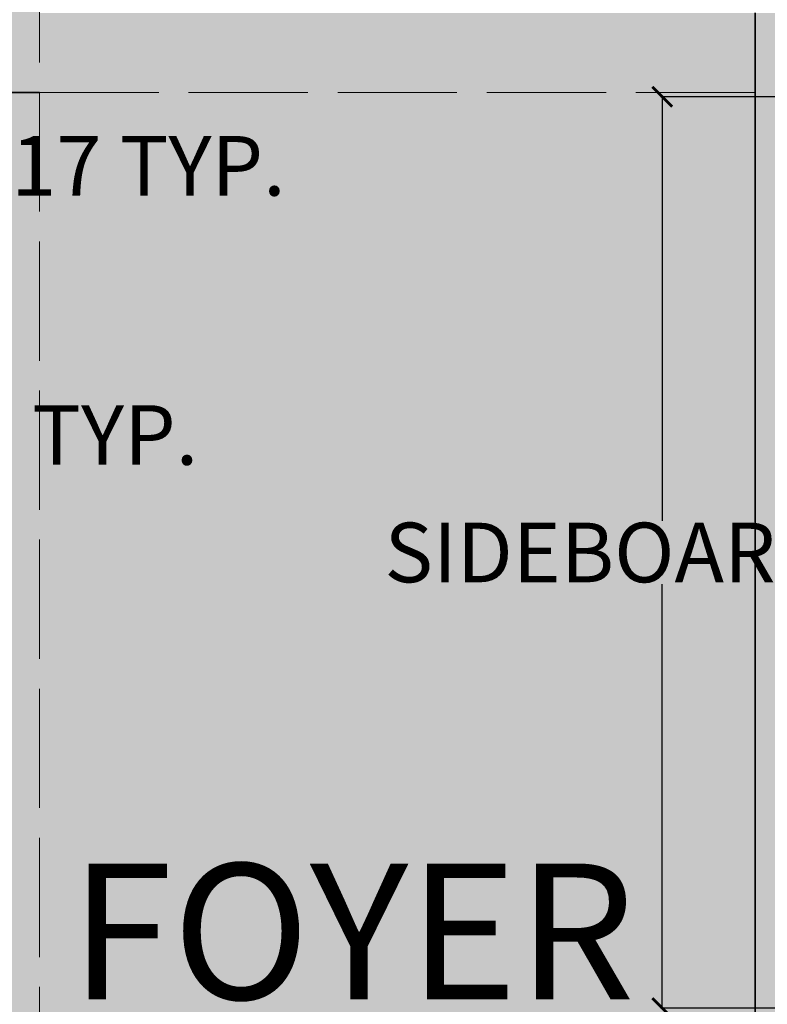
# Model space of a CAD drawing. Units: inches. Extents: x 1704 to 6393, y -157 to 1172.
# Tile 26 of 122: x 2275 to 2351, y 272 to 372. Entities that reach past the tile are written whole.
import ezdxf

# ---------------------------------------------------------------- set-up
doc = ezdxf.new("R2010")
doc.units = ezdxf.units.IN
doc.header["$MEASUREMENT"] = 0
doc.linetypes.add('ACAD_ISO02W100', pattern=[15, 12, -3])
for name, color, linetype, lineweight in [('A-ANNO-DIMS', 7, 'Continuous', 13), ('A-AREA-IDEN', 7, 'Continuous', 18), ('A-WALL-OVHD', 8, 'ACAD_ISO02W100', 13), ('A-WALL-PATT', 7, 'Continuous', 13), ('WALLS', 7, 'Continuous', 35)]:
    doc.layers.add(name, color=color, linetype=linetype, lineweight=lineweight)
doc.layers.add('A-FLOR-PATT', color=7, linetype='Continuous', lineweight=13, true_color=0xf2f2f2)
doc.layers.add('L-HRDS-PATT', color=9, linetype='Continuous', lineweight=13, true_color=0xc5c1ba)
doc.styles.get("Standard").update_dxf_attribs({"font": 'arial.ttf'})
doc.dimstyles.get("Standard").update_dxf_attribs({"dimtxt": 6, "dimasz": 2, "dimexe": 0.18, "dimexo": 0.0625, "dimgap": 0.09, "dimtad": 0, "dimtih": 1, "dimtoh": 1, "dimdec": 1, "dimzin": 0, "dimdsep": 46, "dimlunit": 3, "dimtxsty": 'Standard', "dimblk": 'ARCHTICK', "dimcen": 0.09, "dimadec": 0, "dimazin": 0, "dimtfac": 1, "dimtdec": 1, "dimtofl": 0, "dimtmove": 0, "dimatfit": 3, "dimfxl": 1, "dimtolj": 1, "dimtzin": 0, "dimarcsym": 0})

# ---------------------------------------------------------------- blocks, each defined once
blk = doc.blocks.new('_ArchTick')
at = {"color": 0, "linetype": 'ByBlock', "const_width": 0.15}
blk.add_lwpolyline([(-0.5, -0.5), (0.5, 0.5)], dxfattribs=at)
blk = doc.blocks.new('*D58')
at = {"layer": 'A-ANNO-DIMS', "color": 0, "lineweight": -2, "transparency": 16777216}
for p, q in [((2200.535, 354.321), (2200.535, 357.001)), ((2200.535, 356.821), (2217.621, 356.821)), ((2217.621, 354.321), (2217.621, 357.001)), ((2217.621, 356.821), (2219.621, 356.821))]:
    blk.add_line(p, q, dxfattribs=at)
at = {"layer": 'Defpoints', "color": 0, "lineweight": -3, "transparency": 16777216}
for p in [(2217.621, 356.821), (2200.535, 354.258), (2217.621, 354.258)]:
    blk.add_point(p, dxfattribs=at)
at = {"layer": 'A-ANNO-DIMS', "color": 0, "lineweight": -2, "transparency": 16777216, "xscale": 2, "yscale": 2, "zscale": 2, "rotation": 180}
blk.add_blockref('_ArchTick', (2200.535, 356.821), dxfattribs=at)
at = {"layer": 'A-ANNO-DIMS', "color": 0, "lineweight": -2, "transparency": 16777216, "xscale": 2, "yscale": 2, "zscale": 2}
blk.add_blockref('_ArchTick', (2217.621, 356.821), dxfattribs=at)
at = {"layer": 'A-ANNO-DIMS', "color": 0, "transparency": 16777216, "insert": (2262.58, 356.821), "char_height": 6, "attachment_point": 5}
blk.add_mtext('\\A1;PALLA CHAIR 17 TYP.', dxfattribs=at)
blk = doc.blocks.new('*D62')
at = {"layer": 'A-ANNO-DIMS', "color": 0, "lineweight": -2, "transparency": 16777216}
for p, q in [((2163.814, 333.596), (2163.814, 329.559)), ((2189.944, 333.596), (2189.944, 329.559)), ((2163.814, 329.739), (2189.944, 329.739)), ((2189.944, 329.739), (2191.944, 329.739))]:
    blk.add_line(p, q, dxfattribs=at)
at = {"layer": 'Defpoints', "color": 0, "lineweight": -3, "transparency": 16777216}
for p in [(2163.814, 333.658), (2189.944, 333.658), (2189.944, 329.739)]:
    blk.add_point(p, dxfattribs=at)
at = {"layer": 'A-ANNO-DIMS', "color": 0, "lineweight": -2, "transparency": 16777216, "xscale": 2, "yscale": 2, "zscale": 2, "rotation": 180}
blk.add_blockref('_ArchTick', (2163.814, 329.739), dxfattribs=at)
at = {"layer": 'A-ANNO-DIMS', "color": 0, "lineweight": -2, "transparency": 16777216, "xscale": 2, "yscale": 2, "zscale": 2}
blk.add_blockref('_ArchTick', (2189.944, 329.739), dxfattribs=at)
at = {"layer": 'A-ANNO-DIMS', "color": 0, "transparency": 16777216, "insert": (2244.46, 329.739), "char_height": 6, "attachment_point": 5}
blk.add_mtext('\\A1;BIQUISTEN CHAIR 26 TYP.', dxfattribs=at)
blk = doc.blocks.new('*D68')
at = {"layer": 'A-ANNO-DIMS', "color": 0, "lineweight": -2, "transparency": 16777216}
for p, q in [((2353.706, 363.767), (2339.834, 363.767)), ((2340.014, 363.767), (2340.014, 321.111)), ((2340.014, 272.066), (2340.014, 314.722)), ((2353.706, 272.066), (2339.834, 272.066))]:
    blk.add_line(p, q, dxfattribs=at)
at = {"layer": 'Defpoints', "color": 0, "lineweight": -3, "transparency": 16777216}
for p in [(2340.014, 363.767), (2353.769, 363.767), (2353.769, 272.066)]:
    blk.add_point(p, dxfattribs=at)
at = {"layer": 'A-ANNO-DIMS', "color": 0, "lineweight": -2, "transparency": 16777216, "xscale": 2, "yscale": 2, "zscale": 2}
for p, rotation in [((2340.014, 363.767), 90), ((2340.014, 272.066), 270)]:
    blk.add_blockref('_ArchTick', p, dxfattribs=dict(at, rotation=rotation))
at = {"layer": 'A-ANNO-DIMS', "color": 0, "transparency": 16777216, "insert": (2340.014, 317.916), "char_height": 6, "attachment_point": 5}
blk.add_mtext('\\A1;SIDEBOARD 92', dxfattribs=at)
blk = doc.blocks.new('*D93')
at = {"layer": 'A-ANNO-DIMS', "color": 0, "lineweight": -2, "transparency": 16777216}
for p, q in [((2605.286, 895.213), (1829.698, 895.213)), ((1829.878, 895.213), (1829.878, 495.866)), ((1829.878, 90.213), (1829.878, 489.56)), ((2605.286, 90.213), (1829.698, 90.213))]:
    blk.add_line(p, q, dxfattribs=at)
at = {"layer": 'Defpoints', "color": 0, "lineweight": -3, "transparency": 16777216}
for p in [(2605.349, 895.213), (1829.878, 90.213), (2605.349, 90.213)]:
    blk.add_point(p, dxfattribs=at)
at = {"layer": 'A-ANNO-DIMS', "color": 0, "lineweight": -2, "transparency": 16777216, "xscale": 2, "yscale": 2, "zscale": 2}
for p, rotation in [((1829.878, 895.213), 90), ((1829.878, 90.213), 270)]:
    blk.add_blockref('_ArchTick', p, dxfattribs=dict(at, rotation=rotation))
at = {"layer": 'A-ANNO-DIMS', "color": 0, "transparency": 16777216, "insert": (1829.878, 492.713), "char_height": 6, "attachment_point": 5}
blk.add_mtext('\\A1;805', dxfattribs=at)

msp = doc.modelspace()

# ---------------------------------------------------------------- hatches: boundary and pattern name
at = {"layer": 'A-FLOR-PATT', "transparency": 33554528}
h = msp.add_hatch(color=256, dxfattribs=at)
h.dxf.hatch_style = 1
h.paths.add_polyline_path([(2349.349, 372.213), (2277.349, 372.213), (2277.349, 364.213), (2349.349, 364.213)])
h.paths.add_polyline_path([(2277.349, 372.213), (2273.349, 372.213), (2273.349, 364.213), (2277.349, 364.213)])
h.paths.add_polyline_path([(2277.349, 364.213), (2273.349, 364.213), (2273.349, 202.213), (2277.349, 202.213)])
h.paths.add_polyline_path([(2277.349, 538.213), (2273.349, 538.213), (2273.349, 372.213), (2277.349, 372.213)])
h.paths.add_polyline_path([(2277.349, 629.213), (2273.349, 629.213), (2273.349, 545.213), (2277.349, 545.213)])
h.paths.add_polyline_path([(2277.349, 711.213), (2273.349, 711.213), (2273.349, 631.213), (2277.349, 631.213)])
h.paths.add_polyline_path([(2277.349, 631.213), (2273.349, 631.213), (2273.349, 629.213), (2277.349, 629.213)])
at = {"layer": 'A-WALL-PATT', "transparency": 33554643}
h = msp.add_hatch(color=256, dxfattribs=at)
h.dxf.hatch_style = 1
h.paths.add_polyline_path([(2167.349, 895.213), (2073.349, 895.213), (2073.349, 887.213), (2081.349, 887.213), (2167.349, 887.213)])
h.paths.add_polyline_path([(2465.349, 895.213), (2273.349, 895.213), (2273.349, 903.213), (2263.349, 903.213), (2263.349, 895.213), (2263.349, 887.213), (2325.349, 887.213), (2325.349, 863.213), (2333.349, 863.213), (2333.349, 887.213), (2465.349, 887.213)])
h.paths.add_polyline_path([(2533.349, 895.213), (2513.349, 895.213), (2513.349, 887.213), (2513.349, 861.213), (2517.349, 861.213), (2517.349, 887.213), (2533.349, 887.213)])
h.paths.add_polyline_path([(2605.349, 895.213), (2581.349, 895.213), (2581.349, 887.213), (2597.349, 887.213), (2597.349, 854.213), (2605.349, 854.213)])
h.paths.add_polyline_path([(2605.349, 752.213), (2629.349, 752.213), (2629.349, 716.213), (2605.349, 716.213), (2605.349, 712.213), (2719.349, 712.213), (2719.349, 716.213), (2631.349, 716.213), (2631.349, 754.213), (2605.349, 754.213), (2605.349, 794.213), (2597.349, 794.213), (2597.349, 787.213), (2517.349, 787.213), (2517.349, 813.213), (2513.349, 813.213), (2513.349, 783.213), (2517.349, 783.213), (2597.349, 783.213), (2597.349, 719.213), (2517.349, 719.213), (2517.349, 753.213), (2513.349, 753.213), (2513.349, 719.213), (2365.349, 719.213), (2365.349, 763.213), (2325.349, 763.213), (2325.349, 755.213), (2357.349, 755.213), (2357.349, 719.213), (2325.349, 719.213), (2325.349, 711.213), (2547.349, 711.213), (2547.349, 615.213), (2449.349, 615.213), (2449.349, 607.213), (2514.349, 607.213), (2514.349, 546.213), (2439.349, 546.213), (2425.349, 546.213), (2425.349, 607.213), (2425.349, 615.213), (2350.349, 615.213), (2350.349, 589.713), (2358.349, 589.713), (2358.349, 610.213), (2420.349, 610.213), (2420.349, 545.213), (2358.349, 545.213), (2358.349, 565.713), (2350.349, 565.713), (2350.349, 538.213), (2469.349, 538.213), (2469.349, 459.213), (2469.349, 372.213), (2423.349, 372.213), (2423.349, 364.213), (2473.349, 364.213), (2473.349, 318.213), (2477.349, 318.213), (2477.349, 364.213), (2547.349, 364.213), (2547.349, 352.213), (2549.349, 352.213), (2549.349, 364.213), (2597.349, 364.213), (2597.349, 328.213), (2549.349, 328.213), (2547.349, 328.213), (2547.349, 326.213), (2549.349, 326.213), (2597.349, 326.213), (2605.349, 326.213), (2605.349, 377.057), (2597.349, 377.057), (2597.349, 372.213), (2477.349, 372.213), (2477.349, 451.213), (2597.349, 451.213), (2605.349, 451.213), (2605.349, 459.213), (2597.349, 459.213), (2477.349, 459.213), (2477.349, 538.213), (2597.349, 538.213), (2597.349, 495.213), (2605.349, 495.213), (2605.349, 512.213), (2631.349, 512.213), (2631.349, 568.213), (2605.349, 568.213), (2605.349, 577.213), (2597.349, 577.213), (2597.349, 542.213), (2518.349, 542.213), (2518.349, 607.213), (2532.349, 607.213), (2605.349, 607.213), (2605.349, 615.213), (2597.349, 615.213), (2551.349, 615.213), (2551.349, 711.213), (2597.349, 711.213), (2597.349, 645.213), (2605.349, 645.213), (2605.349, 712.213), (2605.349, 716.213)])
h.paths.add_polyline_path([(2605.349, 566.213), (2629.349, 566.213), (2629.349, 514.213), (2605.349, 514.213)], flags=16)
h.paths.add_polyline_path([(2381.349, 372.213), (2349.349, 372.213), (2349.349, 202.213), (2337.349, 202.213), (2337.349, 194.213), (2349.349, 194.213), (2349.349, 90.213), (2349.349, 72.213), (2357.349, 72.213), (2357.349, 90.213), (2381.349, 90.213), (2381.349, 98.213), (2357.349, 98.213), (2357.349, 266.213), (2381.349, 266.213), (2381.349, 270.213), (2353.349, 270.213), (2353.349, 364.213), (2381.349, 364.213)])
h.paths.add_polyline_path([(2605.349, 302.213), (2597.349, 302.213), (2597.349, 270.213), (2477.349, 270.213), (2477.349, 294.213), (2473.349, 294.213), (2473.349, 270.213), (2423.349, 270.213), (2423.349, 266.213), (2597.349, 266.213), (2597.349, 218.213), (2605.349, 218.213)])
h.paths.add_polyline_path([(2605.349, 146.213), (2597.349, 146.213), (2597.349, 98.213), (2429.349, 98.213), (2429.349, 90.213), (2597.349, 90.213), (2597.349, 72.213), (2605.349, 72.213), (2605.349, 90.213)])
h.paths.add_polyline_path([(2225.349, 202.213), (2049.349, 202.213), (2049.349, 194.213), (2225.349, 194.213)])
h.paths.add_polyline_path([(2289.349, 202.213), (2277.349, 202.213), (2273.349, 202.213), (2269.516, 202.213), (2269.516, 194.213), (2273.349, 194.213), (2277.349, 194.213), (2289.349, 194.213)])
h.paths.add_polyline_path([(2273.349, 372.213), (2029.19, 372.213), (2029.19, 364.213), (2273.349, 364.213)])
h.paths.add_polyline_path([(2277.349, 545.213), (2213.349, 545.213), (2213.349, 573.213), (2205.349, 573.213), (2177.349, 573.213), (2177.349, 545.213), (2073.349, 545.213), (2073.349, 538.213), (2081.349, 538.213), (2277.349, 538.213)])
h.paths.add_polyline_path([(2181.349, 545.213), (2181.349, 569.213), (2205.349, 569.213), (2205.349, 545.213)], flags=16)
h.paths.add_polyline_path([(2277.349, 719.213), (2081.349, 719.213), (2073.349, 719.213), (2073.349, 711.213), (2154.575, 711.213), (2205.349, 711.213), (2205.349, 687.213), (2205.349, 629.213), (2213.349, 629.213), (2273.349, 629.213), (2273.349, 631.213), (2207.349, 631.213), (2207.349, 707.213), (2231.349, 707.213), (2231.349, 709.213), (2207.349, 709.213), (2207.349, 711.213), (2277.349, 711.213)])
at = {"layer": 'L-HRDS-PATT', "transparency": 33554539}
h = msp.add_hatch(color=256, dxfattribs=at)
h.dxf.hatch_style = 1
h.paths.add_polyline_path([(2651.217, 368.213), (2605.349, 368.213), (2605.349, 218.213), (2605.349, 212.464), (2605.349, 210.513), (2605.349, 153.913), (2605.349, 151.962), (2605.349, 146.213), (2605.349, 90.213), (2605.349, 72.213), (2601.349, 72.213), (2600.88, 50.634), (2719.349, 50.634), (2719.349, 72.213), (2711.349, 72.213), (2663.217, 72.213), (2651.217, 72.213)])
h.paths.add_polyline_path([(2711.349, 48.634), (2600.88, 48.634), (2576.88, 48.634), (2576.88, 17.658), (2711.349, 17.658)])
h.paths.add_polyline_path([(2601.349, 72.213), (2597.349, 72.213), (2597.349, 90.213), (2429.349, 90.213), (2425.516, 90.213), (2424.215, 90.213), (2386.482, 90.213), (2385.181, 90.213), (2381.349, 90.213), (2357.349, 90.213), (2357.349, 72.213), (2349.349, 72.213), (2349.349, 90.213), (2349.349, 134.213), (2277.349, 134.213), (2277.349, 50.634), (2566.88, 50.634), (2600.88, 50.634)])
h.paths.add_polyline_path([(2349.349, 146.213), (2277.349, 146.213), (2277.349, 134.213), (2349.349, 134.213)])
h.paths.add_polyline_path([(2349.349, 158.213), (2277.349, 158.213), (2277.349, 146.213), (2349.349, 146.213)])
h.paths.add_polyline_path([(2349.349, 170.213), (2277.349, 170.213), (2277.349, 158.213), (2349.349, 158.213)])
h.paths.add_polyline_path([(2349.349, 194.213), (2337.349, 194.213), (2337.349, 202.213), (2349.349, 202.213), (2349.349, 364.213), (2277.349, 364.213), (2277.349, 202.213), (2289.349, 202.213), (2289.349, 194.213), (2277.349, 194.213), (2277.349, 170.213), (2349.349, 170.213)])

# ---------------------------------------------------------------- linework, layer by layer
at = {"layer": 'A-WALL-OVHD'}
for p, q in [((2277.349, 202.213), (2277.349, 711.213)), ((2277.349, 364.213), (2349.349, 364.213))]:
    msp.add_line(p, q, dxfattribs=at)
at = {"layer": 'WALLS'}
for p, q in [((2349.349, 202.213), (2349.349, 372.213)), ((2277.349, 364.213), (2029.19, 364.213))]:
    msp.add_line(p, q, dxfattribs=at)

# ---------------------------------------------------------------- texts
at = {"layer": 'A-AREA-IDEN'}
msp.add_text('FOYER', height=13.6672, dxfattribs=at).set_placement((2280.423, 272.95))

# ---------------------------------------------------------------- dimensions: what is measured, and where the dimension line sits
at = {"layer": 'A-ANNO-DIMS'}
dim = msp.add_linear_dim(base=(1829.878, 90.213), p1=(2605.349, 895.213), p2=(2605.349, 90.213), angle=90, dimstyle='Standard', override={"dimdec": 0, "dimlfac": 1, "dimrnd": 0, "dimzin": 0, "dimdsep": 46, "dimlunit": 2}, dxfattribs=at)
dim.commit()
dim.dimension.update_dxf_attribs({"geometry": '*D93', "text_midpoint": (1829.878, 492.713)})
for base, p1, p2, text, picture, middle in [((2217.621, 356.821), (2200.535, 354.258), (2217.621, 354.258), 'PALLA CHAIR <> TYP.', '*D58', (2262.58, 356.821)), ((2189.944, 329.739), (2163.814, 333.658), (2189.944, 333.658), 'BIQUISTEN CHAIR <> TYP.', '*D62', (2244.46, 329.739))]:
    dim = msp.add_linear_dim(base=base, p1=p1, p2=p2, text=text, dimstyle='Standard', override={"dimdec": 0, "dimlfac": 1, "dimrnd": 0, "dimzin": 0, "dimdsep": 46, "dimlunit": 2}, dxfattribs=at)
    dim.commit()
    dim.dimension.update_dxf_attribs({"geometry": picture, "text_midpoint": middle})
dim = msp.add_linear_dim(base=(2340.014, 363.767), p1=(2353.769, 272.066), p2=(2353.769, 363.767), angle=90, text='SIDEBOARD <>', dimstyle='Standard', override={"dimdec": 0, "dimlfac": 1, "dimrnd": 0, "dimzin": 0, "dimdsep": 46, "dimlunit": 2}, dxfattribs=at)
dim.commit()
dim.dimension.update_dxf_attribs({"geometry": '*D68', "text_midpoint": (2340.014, 317.916)})

doc.saveas('drawing.dxf')
